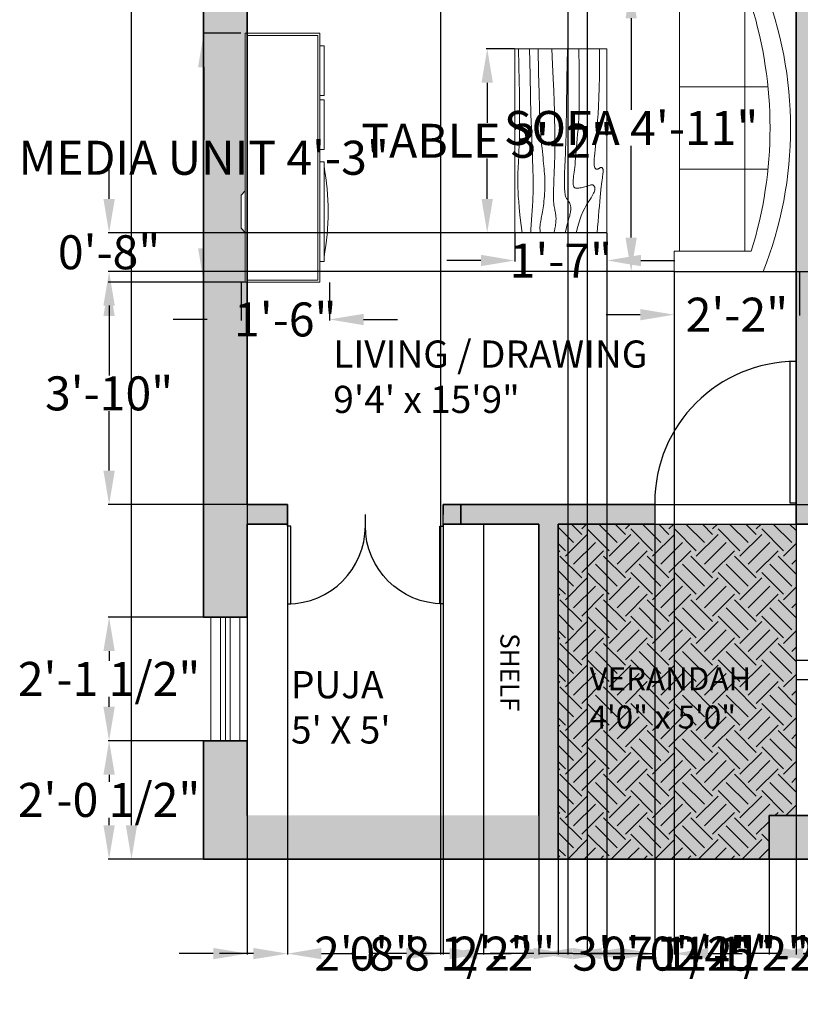
# Model space of a CAD drawing. Units: inches. Extents: x -8 to 329, y 10 to 430.
# Tile 1 of 4: x -8 to 153, y 10 to 213. Entities that reach past the tile are written whole.
import ezdxf

# ---------------------------------------------------------------- set-up
doc = ezdxf.new("R2010")
doc.units = ezdxf.units.IN
doc.header["$MEASUREMENT"] = 0
for name, color, linetype, lineweight in [('A-ANNO-DIMS', 2, 'Continuous', 18), ('A-ANNO-TEXT', 7, 'Continuous', 18), ('A-AREA-IDEN', 7, 'Continuous', 18), ('A-DOOR', 3, 'Continuous', 25), ('A-FLOR-CASE', 9, 'Continuous', 25), ('A-FLOR-STRS', 7, 'Continuous', 25), ('A-FURN', 8, 'Continuous', 18), ('A-GLAZ', 4, 'Continuous', 18), ('A-WALL', 7, 'Continuous', 35), ('A-WALL-PATT', 253, 'Continuous', 13)]:
    doc.layers.add(name, color=color, linetype=linetype, lineweight=lineweight)
doc.layers.add('A-FLOR-BASE-PATT', color=126, linetype='Continuous', lineweight=13, true_color=0x1e6f63)
doc.layers.add('A-FLOR-PATT', color=39, linetype='Continuous', lineweight=13, true_color=0x603913)
doc.styles.get("Standard").update_dxf_attribs({"font": 'arial.ttf'})
doc.dimstyles.get("Standard").update_dxf_attribs({"dimtxt": 7, "dimasz": 7, "dimexe": 0.18, "dimexo": 0.0625, "dimgap": 0.09, "dimtad": 0, "dimtih": 1, "dimtoh": 1, "dimdec": 0, "dimzin": 0, "dimdsep": 46, "dimlunit": 3, "dimtxsty": 'Standard', "dimcen": 0.09, "dimadec": 0, "dimazin": 0, "dimtfac": 1, "dimtdec": 0, "dimtofl": 0, "dimtmove": 0, "dimatfit": 3, "dimfxl": 1, "dimtolj": 1, "dimtzin": 0, "dimarcsym": 0})

# ---------------------------------------------------------------- blocks, each defined once
blk = doc.blocks.new('Sofa - Roundback 7 ft.')
for p, q in [((-12.00002, -32.4421), (-12.00003, -6.5971)), ((11.99997, -32.4421), (11.99998, -6.5971)), ((-36.000027, -34), (-36.000027, -11.4696)), ((35.99998, -34), (35.99998, -11.4696)), ((-35.999844, -13.3819), (35.9998, -13.3819)), ((-36.000027, -32.4421), (35.99998, -32.4421))]:
    blk.add_line(p, q)
for points in [[(-36.000027, -34), (-42.000027, -34), (-42.000027, -8)], [(41.99998, -8), (41.99998, -34), (35.99998, -34)]]:
    blk.add_lwpolyline(points)
for centre, radius, start, end in [((0, -114.25), 114.25, 68.43141, 111.5686), ((-0.00001, -127.1968), 121.1968, 72.72033, 107.2797)]:
    blk.add_arc(centre, radius, start, end)
blk = doc.blocks.new('Entertainment Center')
for p, q in [((-4, 0), (-5, -1)), ((4, 0), (-4, 0)), ((5, -1), (4, 0)), ((-17, -19), (-17, -1)), ((-17, -1), (43, -1)), ((-16.5, -18.5), (-16.5, -1.5)), ((-16.5, -1.5), (42.5, -1.5)), ((42.5, -1.5), (42.5, -18.5)), ((43, -1), (43, -19)), ((42.5, -18.5), (-16.5, -18.5)), ((43, -19), (-17, -19)), ((-12, -20), (-12, -19)), ((12, -20), (-12, -20)), ((12, -19), (12, -20)), ((15, -20), (15, -19)), ((27, -20), (15, -20)), ((27, -19), (27, -20)), ((28, -20), (28, -19)), ((40, -20), (28, -20)), ((40, -19), (40, -20))]:
    blk.add_line(p, q)
blk.add_arc((0, 40), 61, 259.6111, 280.3889)
blk = doc.blocks.new('Table - Rectangular Woodgrain 60 x 30 in.')
for p, q in [((0, 0), (0, -30)), ((60, 0), (0, 0)), ((60, -30), (60, 0)), ((0, -30), (60, -30))]:
    blk.add_line(p, q)
for points in [[(0, -2.4), (4.8155, -2.418), (9.0302, -2.4688), (12.709, -2.5477), (15.9167, -2.65), (18.7181, -2.7711), (21.1781, -2.9063), (23.3616, -3.0508), (25.3333, -3.2), (27.1477, -3.3495), (28.8172, -3.4958), (30.3437, -3.636), (31.7291, -3.7667), (32.9756, -3.8849), (34.0849, -3.9875), (35.059, -4.0714), (35.9, -4.1334), (36.6114, -4.1711), (37.2041, -4.1854), (37.6906, -4.1779), (38.0833, -4.15), (38.3948, -4.1034), (38.6375, -4.0396), (38.8239, -3.9602), (38.9666, -3.8667), (39.0764, -3.7608), (39.1573, -3.6448), (39.2116, -3.521), (39.2416, -3.3917), (39.2498, -3.2593), (39.2385, -3.1261), (39.21, -2.9944), (39.1666, -2.8667), (39.111, -2.7447), (39.0468, -2.6281), (38.978, -2.5163), (38.9083, -2.4083), (38.8418, -2.3035), (38.7823, -2.201), (38.7337, -2.1001), (38.7, -2), (38.6844, -1.9003), (38.6875, -1.8021), (38.7094, -1.707), (38.75, -1.6167), (38.8094, -1.5326), (38.8875, -1.4563), (38.9844, -1.3893), (39.1, -1.3333), (39.2351, -1.2896), (39.3937, -1.2583), (39.5804, -1.2396), (39.8, -1.2333), (40.057, -1.2396), (40.3562, -1.2583), (40.7023, -1.2896), (41.1, -1.3333), (41.5547, -1.3895), (42.0755, -1.4573), (42.6721, -1.5361), (43.3542, -1.625), (44.1316, -1.7233), (45.014, -1.8302), (46.0114, -1.9449), (47.1333, -2.0667), (48.3862, -2.1947), (49.7625, -2.3281), (51.2513, -2.4663), (52.8416, -2.6083), (54.5226, -2.7535), (56.2833, -2.9011), (58.1127, -3.0501), (60, -3.2)], [(0, -9.2), (6.5759, -9.0858), (11.9385, -9.0365), (16.2527, -9.0418), (19.6833, -9.0917), (22.3952, -9.1759), (24.5531, -9.2844), (26.322, -9.4069), (27.8666, -9.5333), (29.3241, -9.6553), (30.7203, -9.7719), (32.0532, -9.8837), (33.3208, -9.9917), (34.5213, -10.0965), (35.6526, -10.199), (36.7128, -10.2999), (37.7, -10.4), (38.6129, -10.4996), (39.4531, -10.5969), (40.223, -10.6895), (40.925, -10.775), (41.5613, -10.8512), (42.1344, -10.9156), (42.6465, -10.966), (43.1, -11), (43.4976, -11.0158), (43.8437, -11.0136), (44.143, -10.9942), (44.4, -10.9583), (44.6195, -10.9069), (44.8062, -10.8406), (44.9648, -10.7603), (45.1, -10.6667), (45.2155, -10.5598), (45.3114, -10.4365), (45.3871, -10.2929), (45.4416, -10.125), (45.4743, -9.929), (45.4844, -9.7011), (45.4709, -9.4371), (45.4333, -9.1333), (45.3716, -8.7883), (45.2896, -8.4104), (45.1919, -8.0107), (45.0833, -7.6), (44.9685, -7.1893), (44.8521, -6.7896), (44.7388, -6.4117), (44.6333, -6.0667), (44.54, -5.7628), (44.4614, -5.4979), (44.4001, -5.2675), (44.3583, -5.0667), (44.3384, -4.8909), (44.3427, -4.7354), (44.3736, -4.5956), (44.4333, -4.4667), (44.5236, -4.3453), (44.6427, -4.2333), (44.7884, -4.1339), (44.9583, -4.05), (45.1501, -3.9849), (45.3614, -3.9417), (45.59, -3.9234), (45.8333, -3.9333), (46.0915, -3.9749), (46.3734, -4.0531), (46.6906, -4.1736), (47.0542, -4.3417), (47.4756, -4.5629), (47.9661, -4.8427), (48.5372, -5.1866), (49.2, -5.6), (49.9676, -6.0844), (50.8594, -6.625), (51.8965, -7.2031), (53.1, -7.8), (54.491, -8.3969), (56.0906, -8.975), (57.9199, -9.5156), (60, -10)], [(0, -12.8), (5.1847, -12.9322), (9.6213, -13.0323), (13.3963, -13.1059), (16.5958, -13.1583), (19.3063, -13.1952), (21.614, -13.2219), (23.6054, -13.2439), (25.3666, -13.2667), (26.9728, -13.2947), (28.4531, -13.3281), (29.8256, -13.3663), (31.1083, -13.4083), (32.3191, -13.4535), (33.476, -13.501), (34.597, -13.5501), (35.7, -13.6), (36.7984, -13.6497), (37.8875, -13.6979), (38.9578, -13.743), (40, -13.7833), (41.0047, -13.8174), (41.9625, -13.8438), (42.864, -13.8607), (43.7, -13.8667), (44.4631, -13.8604), (45.1552, -13.8417), (45.7801, -13.8104), (46.3416, -13.7667), (46.8439, -13.7104), (47.2906, -13.6417), (47.6858, -13.5604), (48.0333, -13.4667), (48.3375, -13.3608), (48.6042, -13.2448), (48.8396, -13.121), (49.05, -12.9917), (49.2417, -12.8593), (49.4208, -12.7261), (49.5937, -12.5944), (49.7667, -12.4667), (49.9452, -12.3451), (50.1323, -12.2313), (50.3303, -12.1268), (50.5416, -12.0333), (50.7686, -11.9524), (51.0135, -11.8854), (51.2788, -11.8341), (51.5666, -11.8), (51.8785, -11.7843), (52.2116, -11.7865), (52.562, -11.8059), (52.926, -11.8417), (53.2998, -11.8931), (53.6795, -11.9594), (54.0614, -12.0397), (54.4416, -12.1333), (54.8223, -12.2401), (55.2293, -12.3625), (55.6942, -12.5037), (56.2489, -12.6667), (56.9251, -12.8547), (57.7545, -13.0708), (58.7689, -13.3182), (60, -13.6)], [(0, -18), (5.124, -17.7273), (9.6609, -17.5057), (13.6705, -17.3303), (17.2125, -17.1958), (20.3467, -17.0973), (23.1328, -17.0297), (25.6307, -16.9878), (27.9, -16.9667), (29.9928, -16.9617), (31.9302, -16.9703), (33.7254, -16.9907), (35.3917, -17.0208), (36.9423, -17.0588), (38.3906, -17.1026), (39.7499, -17.1503), (41.0333, -17.2), (42.2519, -17.2496), (43.4073, -17.2969), (44.4986, -17.3395), (45.525, -17.375), (46.4858, -17.4012), (47.3802, -17.4156), (48.2074, -17.416), (48.9667, -17.4), (49.6583, -17.3662), (50.2872, -17.3167), (50.8595, -17.2547), (51.3812, -17.1833), (51.8584, -17.1057), (52.2971, -17.025), (52.7034, -16.9443), (53.0833, -16.8667), (53.443, -16.7951), (53.789, -16.7313), (54.128, -16.6768), (54.4666, -16.6334), (54.8115, -16.6024), (55.1693, -16.5854), (55.5465, -16.5841), (55.95, -16.6), (56.3828, -16.6337), (56.8346, -16.6823), (57.2915, -16.7418), (57.7396, -16.8084), (58.165, -16.878), (58.5539, -16.9469), (58.8924, -17.0111), (59.1666, -17.0667), (59.3679, -17.1107), (59.5078, -17.1438), (59.6032, -17.1675), (59.6708, -17.1833), (59.7275, -17.193), (59.7901, -17.1979), (59.8753, -17.1998), (60, -17.2)], [(0, -22.4), (8.0098, -22.2501), (14.4094, -22.1011), (19.4168, -21.9535), (23.25, -21.8083), (26.1269, -21.6663), (28.2656, -21.5281), (29.884, -21.3947), (31.2, -21.2667), (32.3967, -21.1448), (33.5172, -21.0292), (34.5697, -20.9198), (35.5625, -20.8167), (36.5037, -20.7198), (37.4015, -20.6292), (38.2642, -20.5448), (39.1, -20.4667), (39.9164, -20.3951), (40.7187, -20.3313), (41.5117, -20.2768), (42.3, -20.2333), (43.0883, -20.2024), (43.8812, -20.1854), (44.6836, -20.1841), (45.5, -20.2), (46.3328, -20.234), (47.1747, -20.2844), (48.0163, -20.3488), (48.8479, -20.425), (49.66, -20.5106), (50.4429, -20.6031), (51.1872, -20.7004), (51.8833, -20.8), (52.5246, -20.8999), (53.1166, -20.9995), (53.6681, -21.0983), (54.1875, -21.1958), (54.6834, -21.2919), (55.1646, -21.3859), (55.6394, -21.4777), (56.1167, -21.5667), (56.6028, -21.6515), (57.0961, -21.7266), (57.5929, -21.7852), (58.0896, -21.8208), (58.5823, -21.8268), (59.0674, -21.7964), (59.5412, -21.723), (60, -21.6)], [(0, -25.2), (8.6355, -25.0504), (15.7026, -24.9031), (21.4049, -24.7606), (25.9458, -24.625), (29.529, -24.4988), (32.3578, -24.3844), (34.6359, -24.284), (36.5667, -24.2), (38.3213, -24.1341), (39.9417, -24.0854), (41.437, -24.0523), (42.8167, -24.0333), (44.0901, -24.0268), (45.2667, -24.0313), (46.3557, -24.0451), (47.3667, -24.0667), (48.309, -24.0947), (49.1928, -24.1287), (50.0284, -24.168), (50.826, -24.2125), (51.5959, -24.2617), (52.3483, -24.3151), (53.0935, -24.3725), (53.8417, -24.4334), (54.6009, -24.497), (55.3699, -24.561), (56.1454, -24.6226), (56.9239, -24.6792), (57.7021, -24.7279), (58.4764, -24.7662), (59.2435, -24.7911), (60, -24.8)], [(0, -28.8), (5.6867, -28.6681), (10.45, -28.5698), (14.407, -28.5012), (17.675, -28.4584), (20.3711, -28.4374), (22.6125, -28.4344), (24.5164, -28.4455), (26.2, -28.4667), (27.762, -28.4947), (29.2276, -28.5281), (30.6033, -28.5663), (31.8958, -28.6084), (33.1118, -28.6535), (34.2578, -28.7011), (35.3405, -28.7501), (36.3666, -28.8), (37.3443, -28.8497), (38.288, -28.8974), (39.2137, -28.9412), (40.1375, -28.9792), (41.0753, -29.0093), (42.0432, -29.0297), (43.0572, -29.0384), (44.1333, -29.0333), (45.2936, -29.0114), (46.5843, -28.9641), (48.0579, -28.8816), (49.7666, -28.7542), (51.7629, -28.5721), (54.0989, -28.3255), (56.8272, -28.0048), (60, -27.6)]]:
    blk.add_lwpolyline(points)
blk = doc.blocks.new('*U11')
for p, q in [((0, 0), (0, 6)), ((40, 0), (40, 6))]:
    blk.add_line(p, q)
blk.add_lwpolyline([(0, 0), (0, -40), (1.75, -40), (1.75, 0)], close=True)
blk.add_arc((0, 0), 40, 270, 0)
blk = doc.blocks.new('*U12')
for p, q in [((0, 0), (0, -6)), ((-40, 0), (-40, -6))]:
    blk.add_line(p, q)
blk.add_lwpolyline([(0, 0), (0, 40), (-1.75, 40), (-1.75, 0)], close=True)
blk.add_arc((0, 0), 40, 90, 180)
blk = doc.blocks.new('*D15')
at = {"layer": 'A-ANNO-DIMS', "color": 0, "lineweight": -2, "transparency": 16777216}
for p, q in [((29.84, 399.76), (14.88, 399.76)), ((15.06, 392.76), (15.06, 223.43)), ((15.06, 46.76), (15.06, 216.1)), ((29.84, 39.76), (14.88, 39.76))]:
    blk.add_line(p, q, dxfattribs=at)
at = {"layer": 'A-ANNO-DIMS', "color": 0, "transparency": 16777216}
for points in [[(13.89, 392.76), (16.23, 392.76), (15.06, 399.76)], [(13.89, 46.76), (16.23, 46.76), (15.06, 39.76)]]:
    blk.add_solid(points, dxfattribs=at)
at = {"layer": 'Defpoints', "color": 0, "transparency": 16777216}
for p in [(29.9, 399.76), (15.06, 39.76), (29.9, 39.76)]:
    blk.add_point(p, dxfattribs=at)
at = {"layer": 'A-ANNO-DIMS', "color": 0, "transparency": 16777216, "insert": (15.06, 219.76), "char_height": 7, "attachment_point": 5}
blk.add_mtext('\\A1;30\'0"', dxfattribs=at)
blk = doc.blocks.new('*D32')
at = {"layer": 'A-ANNO-DIMS', "color": 0, "lineweight": -2, "transparency": 16777216}
for p, q in [((126.75, 219.9), (117.76, 219.9)), ((117.94, 212.9), (117.94, 194.03)), ((117.94, 167.75), (117.94, 186.61)), ((126.75, 160.75), (117.76, 160.75))]:
    blk.add_line(p, q, dxfattribs=at)
at = {"layer": 'A-ANNO-DIMS', "color": 0, "transparency": 16777216}
for points in [[(116.77, 212.9), (119.1, 212.9), (117.94, 219.9)], [(116.77, 167.75), (119.1, 167.75), (117.94, 160.75)]]:
    blk.add_solid(points, dxfattribs=at)
at = {"layer": 'Defpoints', "color": 0, "transparency": 16777216}
for p in [(126.81, 219.9), (117.94, 160.75), (126.81, 160.75)]:
    blk.add_point(p, dxfattribs=at)
at = {"layer": 'A-ANNO-DIMS', "color": 0, "transparency": 16777216, "insert": (117.94, 190.32), "char_height": 7, "attachment_point": 5}
blk.add_mtext('\\A1;SOFA 4\'-11"', dxfattribs=at)
blk = doc.blocks.new('*D33')
at = {"layer": 'A-ANNO-DIMS', "color": 0, "lineweight": -2, "transparency": 16777216}
for p, q in [((126.81, 160.68), (126.81, 151.69)), ((152.63, 160.68), (152.63, 151.69)), ((119.81, 151.87), (112.81, 151.87)), ((159.63, 151.87), (166.63, 151.87))]:
    blk.add_line(p, q, dxfattribs=at)
at = {"layer": 'A-ANNO-DIMS', "color": 0, "transparency": 16777216}
for points in [[(119.81, 153.04), (119.81, 150.71), (126.81, 151.87)], [(159.63, 153.04), (159.63, 150.71), (152.63, 151.87)]]:
    blk.add_solid(points, dxfattribs=at)
at = {"layer": 'Defpoints', "color": 0, "transparency": 16777216}
for p in [(126.81, 160.75), (152.63, 160.75), (152.63, 151.87)]:
    blk.add_point(p, dxfattribs=at)
at = {"layer": 'A-ANNO-DIMS', "color": 0, "transparency": 16777216, "insert": (139.72, 151.87), "char_height": 7, "attachment_point": 5}
blk.add_mtext('\\A1;2\'-2"', dxfattribs=at)
blk = doc.blocks.new('*D34')
at = {"layer": 'A-ANNO-DIMS', "color": 0, "lineweight": -2, "transparency": 16777216}
for p, q in [((37.56, 209.81), (29.75, 209.81)), ((29.93, 202.81), (29.93, 187.86)), ((29.93, 165.57), (29.93, 180.52)), ((37.56, 158.57), (29.75, 158.57))]:
    blk.add_line(p, q, dxfattribs=at)
at = {"layer": 'A-ANNO-DIMS', "color": 0, "transparency": 16777216}
for points in [[(28.77, 202.81), (31.1, 202.81), (29.93, 209.81)], [(28.77, 165.57), (31.1, 165.57), (29.93, 158.57)]]:
    blk.add_solid(points, dxfattribs=at)
at = {"layer": 'Defpoints', "color": 0, "transparency": 16777216}
for p in [(29.93, 209.81), (37.62, 209.81), (37.62, 158.57)]:
    blk.add_point(p, dxfattribs=at)
at = {"layer": 'A-ANNO-DIMS', "color": 0, "transparency": 16777216, "insert": (29.93, 184.19), "char_height": 7, "attachment_point": 5}
blk.add_mtext('\\A1;MEDIA UNIT 4\'-3"', dxfattribs=at)
blk = doc.blocks.new('*D35')
at = {"layer": 'A-ANNO-DIMS', "color": 0, "lineweight": -2, "transparency": 16777216}
for p, q in [((37.62, 158.51), (37.62, 150.71)), ((55.84, 158.51), (55.84, 150.71)), ((30.62, 150.89), (23.62, 150.89)), ((62.84, 150.89), (69.84, 150.89))]:
    blk.add_line(p, q, dxfattribs=at)
at = {"layer": 'A-ANNO-DIMS', "color": 0, "transparency": 16777216}
for points in [[(30.62, 152.05), (30.62, 149.72), (37.62, 150.89)], [(62.84, 152.05), (62.84, 149.72), (55.84, 150.89)]]:
    blk.add_solid(points, dxfattribs=at)
at = {"layer": 'Defpoints', "color": 0, "transparency": 16777216}
for p in [(37.62, 158.57), (55.84, 158.57), (37.62, 150.89)]:
    blk.add_point(p, dxfattribs=at)
at = {"layer": 'A-ANNO-DIMS', "color": 0, "transparency": 16777216, "insert": (46.73, 150.89), "char_height": 7, "attachment_point": 5}
blk.add_mtext('\\A1;1\'-6"', dxfattribs=at)
blk = doc.blocks.new('*D36')
at = {"layer": 'A-ANNO-DIMS', "color": 0, "lineweight": -2, "transparency": 16777216}
for p, q in [((93.93, 206.64), (88.12, 206.64)), ((88.3, 199.64), (88.3, 191.35)), ((88.3, 175.72), (88.3, 184.01)), ((93.93, 168.72), (88.12, 168.72))]:
    blk.add_line(p, q, dxfattribs=at)
at = {"layer": 'A-ANNO-DIMS', "color": 0, "transparency": 16777216}
for points in [[(87.13, 199.64), (89.47, 199.64), (88.3, 206.64)], [(87.13, 175.72), (89.47, 175.72), (88.3, 168.72)]]:
    blk.add_solid(points, dxfattribs=at)
at = {"layer": 'Defpoints', "color": 0, "transparency": 16777216}
for p in [(93.99, 206.64), (88.3, 168.72), (93.99, 168.72)]:
    blk.add_point(p, dxfattribs=at)
at = {"layer": 'A-ANNO-DIMS', "color": 0, "transparency": 16777216, "insert": (88.3, 187.68), "char_height": 7, "attachment_point": 5}
blk.add_mtext('\\A1;TABLE 3\'-2"', dxfattribs=at)
blk = doc.blocks.new('*D37')
at = {"layer": 'A-ANNO-DIMS', "color": 0, "lineweight": -2, "transparency": 16777216}
for p, q in [((93.99, 168.66), (93.99, 162.85)), ((112.95, 168.66), (112.95, 162.85)), ((86.99, 163.03), (79.99, 163.03)), ((119.95, 163.03), (126.95, 163.03))]:
    blk.add_line(p, q, dxfattribs=at)
at = {"layer": 'A-ANNO-DIMS', "color": 0, "transparency": 16777216}
for points in [[(86.99, 164.2), (86.99, 161.86), (93.99, 163.03)], [(119.95, 164.2), (119.95, 161.86), (112.95, 163.03)]]:
    blk.add_solid(points, dxfattribs=at)
at = {"layer": 'Defpoints', "color": 0, "transparency": 16777216}
for p in [(93.99, 168.72), (112.95, 168.72), (112.95, 163.03)]:
    blk.add_point(p, dxfattribs=at)
at = {"layer": 'A-ANNO-DIMS', "color": 0, "transparency": 16777216, "insert": (103.47, 163.03), "char_height": 7, "attachment_point": 5}
blk.add_mtext('\\A1;1\'-7"', dxfattribs=at)
blk = doc.blocks.new('*D44')
at = {"layer": 'A-ANNO-DIMS', "color": 0, "lineweight": -2, "transparency": 16777216}
for p, q in [((122.79, 108.7), (122.79, 20.13)), ((151.9, 108.7), (151.9, 20.13)), ((115.79, 20.31), (108.79, 20.31)), ((158.9, 20.31), (165.9, 20.31))]:
    blk.add_line(p, q, dxfattribs=at)
at = {"layer": 'A-ANNO-DIMS', "color": 0, "transparency": 16777216}
for points in [[(115.79, 21.48), (115.79, 19.15), (122.79, 20.31)], [(158.9, 21.48), (158.9, 19.15), (151.9, 20.31)]]:
    blk.add_solid(points, dxfattribs=at)
at = {"layer": 'Defpoints', "color": 0, "transparency": 16777216}
for p in [(122.79, 108.76), (151.9, 108.76), (151.9, 20.31)]:
    blk.add_point(p, dxfattribs=at)
at = {"layer": 'A-ANNO-DIMS', "color": 0, "transparency": 16777216, "insert": (137.34, 20.31), "char_height": 7, "attachment_point": 5}
blk.add_mtext('\\A1;2\'-5"', dxfattribs=at)
blk = doc.blocks.new('*D45')
at = {"layer": 'A-ANNO-DIMS', "color": 0, "lineweight": -2, "transparency": 16777216}
for p, q in [((47.18, 108.7), (47.18, 20.13)), ((79.25, 108.7), (79.25, 20.13)), ((40.18, 20.31), (33.18, 20.31)), ((86.25, 20.31), (93.25, 20.31))]:
    blk.add_line(p, q, dxfattribs=at)
at = {"layer": 'A-ANNO-DIMS', "color": 0, "transparency": 16777216}
for points in [[(40.18, 21.48), (40.18, 19.15), (47.18, 20.31)], [(86.25, 21.48), (86.25, 19.15), (79.25, 20.31)]]:
    blk.add_solid(points, dxfattribs=at)
at = {"layer": 'Defpoints', "color": 0, "transparency": 16777216}
for p in [(47.18, 108.76), (79.25, 108.76), (79.25, 20.31)]:
    blk.add_point(p, dxfattribs=at)
at = {"layer": 'A-ANNO-DIMS', "color": 0, "transparency": 16777216, "insert": (63.22, 20.31), "char_height": 7, "attachment_point": 5}
blk.add_mtext('\\A1;2\'-8"', dxfattribs=at)
blk = doc.blocks.new('*D46')
at = {"layer": 'A-ANNO-DIMS', "color": 0, "lineweight": -2, "transparency": 16777216}
for p, q in [((38.9, 112.7), (38.9, 20.13)), ((47.18, 112.7), (47.18, 20.13)), ((31.9, 20.31), (24.9, 20.31)), ((54.18, 20.31), (61.18, 20.31))]:
    blk.add_line(p, q, dxfattribs=at)
at = {"layer": 'A-ANNO-DIMS', "color": 0, "transparency": 16777216}
for points in [[(31.9, 21.48), (31.9, 19.15), (38.9, 20.31)], [(54.18, 21.48), (54.18, 19.15), (47.18, 20.31)]]:
    blk.add_solid(points, dxfattribs=at)
at = {"layer": 'Defpoints', "color": 0, "transparency": 16777216}
for p in [(38.9, 112.76), (47.18, 112.76), (47.18, 20.31)]:
    blk.add_point(p, dxfattribs=at)
at = {"layer": 'A-ANNO-DIMS', "color": 0, "transparency": 16777216, "insert": (78.73, 20.31), "char_height": 7, "attachment_point": 5}
blk.add_mtext('\\A1;0\'-8 1/2"', dxfattribs=at)
blk = doc.blocks.new('*D50')
at = {"layer": 'A-ANNO-DIMS', "color": 0, "lineweight": -2, "transparency": 16777216}
for p, q in [((78.68, 302.7), (78.68, 20.13)), ((104.9, 302.7), (104.9, 20.13)), ((71.68, 20.31), (64.68, 20.31)), ((111.9, 20.31), (118.9, 20.31))]:
    blk.add_line(p, q, dxfattribs=at)
at = {"layer": 'A-ANNO-DIMS', "color": 0, "transparency": 16777216}
for points in [[(71.68, 21.48), (71.68, 19.15), (78.68, 20.31)], [(111.9, 21.48), (111.9, 19.15), (104.9, 20.31)]]:
    blk.add_solid(points, dxfattribs=at)
at = {"layer": 'Defpoints', "color": 0, "transparency": 16777216}
for p in [(78.68, 302.76), (104.9, 302.76), (104.9, 20.31)]:
    blk.add_point(p, dxfattribs=at)
at = {"layer": 'A-ANNO-DIMS', "color": 0, "transparency": 16777216, "insert": (91.79, 20.31), "char_height": 7, "attachment_point": 5}
blk.add_mtext('\\A1;2\'-2"', dxfattribs=at)
blk = doc.blocks.new('*D51')
at = {"layer": 'A-ANNO-DIMS', "color": 0, "lineweight": -2, "transparency": 16777216}
for p, q in [((98.9, 48.7), (98.9, 20.13)), ((87.54, 39.7), (87.54, 20.13)), ((80.54, 20.31), (73.54, 20.31)), ((105.9, 20.31), (112.9, 20.31))]:
    blk.add_line(p, q, dxfattribs=at)
at = {"layer": 'A-ANNO-DIMS', "color": 0, "transparency": 16777216}
for points in [[(80.54, 21.48), (80.54, 19.15), (87.54, 20.31)], [(105.9, 21.48), (105.9, 19.15), (98.9, 20.31)]]:
    blk.add_solid(points, dxfattribs=at)
at = {"layer": 'Defpoints', "color": 0, "transparency": 16777216}
for p in [(98.9, 48.76), (87.54, 39.76), (98.9, 20.31)]:
    blk.add_point(p, dxfattribs=at)
at = {"layer": 'A-ANNO-DIMS', "color": 0, "transparency": 16777216, "insert": (133.17, 20.31), "char_height": 7, "attachment_point": 5}
blk.add_mtext('\\A1;0\'-11 1/2"', dxfattribs=at)
blk = doc.blocks.new('*D54')
at = {"layer": 'A-ANNO-DIMS', "color": 0, "lineweight": -2, "transparency": 16777216}
for p, q in [((29.84, 89.59), (10.27, 89.59)), ((10.45, 82.59), (10.45, 80.58)), ((10.45, 71.15), (10.45, 73.16)), ((29.84, 64.15), (10.27, 64.15))]:
    blk.add_line(p, q, dxfattribs=at)
at = {"layer": 'A-ANNO-DIMS', "color": 0, "transparency": 16777216}
for points in [[(9.28, 82.59), (11.62, 82.59), (10.45, 89.59)], [(9.28, 71.15), (11.62, 71.15), (10.45, 64.15)]]:
    blk.add_solid(points, dxfattribs=at)
at = {"layer": 'Defpoints', "color": 0, "transparency": 16777216}
for p in [(29.9, 89.59), (10.45, 64.15), (29.9, 64.15)]:
    blk.add_point(p, dxfattribs=at)
at = {"layer": 'A-ANNO-DIMS', "color": 0, "transparency": 16777216, "insert": (10.45, 76.87), "char_height": 7, "attachment_point": 5}
blk.add_mtext('\\A1;2\'-1 1/2"', dxfattribs=at)
blk = doc.blocks.new('*D61')
at = {"layer": 'A-ANNO-DIMS', "color": 0, "lineweight": -2, "transparency": 16777216}
for p, q in [((29.84, 64.15), (10.27, 64.15)), ((10.45, 57.15), (10.45, 55.66)), ((10.45, 46.76), (10.45, 48.25)), ((29.84, 39.76), (10.27, 39.76))]:
    blk.add_line(p, q, dxfattribs=at)
at = {"layer": 'A-ANNO-DIMS', "color": 0, "transparency": 16777216}
for points in [[(9.28, 57.15), (11.62, 57.15), (10.45, 64.15)], [(9.28, 46.76), (11.62, 46.76), (10.45, 39.76)]]:
    blk.add_solid(points, dxfattribs=at)
at = {"layer": 'Defpoints', "color": 0, "transparency": 16777216}
for p in [(10.45, 64.15), (29.9, 64.15), (29.9, 39.76)]:
    blk.add_point(p, dxfattribs=at)
at = {"layer": 'A-ANNO-DIMS', "color": 0, "transparency": 16777216, "insert": (10.45, 51.96), "char_height": 7, "attachment_point": 5}
blk.add_mtext('\\A1;2\'-0 1/2"', dxfattribs=at)
blk = doc.blocks.new('*D66')
at = {"layer": 'A-ANNO-DIMS', "color": 0, "lineweight": -2, "transparency": 16777216}
for p, q in [((155.9, 48.7), (155.9, 20.13)), ((164.9, 48.7), (164.9, 20.13)), ((148.9, 20.31), (141.9, 20.31)), ((171.9, 20.31), (178.9, 20.31))]:
    blk.add_line(p, q, dxfattribs=at)
at = {"layer": 'A-ANNO-DIMS', "color": 0, "transparency": 16777216}
for points in [[(148.9, 21.48), (148.9, 19.15), (155.9, 20.31)], [(171.9, 21.48), (171.9, 19.15), (164.9, 20.31)]]:
    blk.add_solid(points, dxfattribs=at)
at = {"layer": 'Defpoints', "color": 0, "transparency": 16777216}
for p in [(155.9, 48.76), (164.9, 48.76), (164.9, 20.31)]:
    blk.add_point(p, dxfattribs=at)
at = {"layer": 'A-ANNO-DIMS', "color": 0, "transparency": 16777216, "insert": (188.29, 20.31), "char_height": 7, "attachment_point": 5}
blk.add_mtext('\\A1;0\'-9"', dxfattribs=at)
blk = doc.blocks.new('*D70')
at = {"layer": 'A-ANNO-DIMS', "color": 0, "lineweight": -2, "transparency": 16777216}
for p, q in [((104.9, 306.7), (104.9, 20.13)), ((108.9, 306.7), (108.9, 20.13)), ((97.9, 20.31), (90.9, 20.31)), ((115.9, 20.31), (122.9, 20.31))]:
    blk.add_line(p, q, dxfattribs=at)
at = {"layer": 'A-ANNO-DIMS', "color": 0, "transparency": 16777216}
for points in [[(97.9, 21.48), (97.9, 19.15), (104.9, 20.31)], [(115.9, 21.48), (115.9, 19.15), (108.9, 20.31)]]:
    blk.add_solid(points, dxfattribs=at)
at = {"layer": 'Defpoints', "color": 0, "transparency": 16777216}
for p in [(104.9, 306.76), (108.9, 306.76), (108.9, 20.31)]:
    blk.add_point(p, dxfattribs=at)
at = {"layer": 'A-ANNO-DIMS', "color": 0, "transparency": 16777216, "insert": (132.29, 20.31), "char_height": 7, "attachment_point": 5}
blk.add_mtext('\\A1;0\'-4"', dxfattribs=at)
blk = doc.blocks.new('*D71')
at = {"layer": 'A-ANNO-DIMS', "color": 0, "lineweight": -2, "transparency": 16777216}
for p, q in [((102.9, 39.7), (102.9, 20.13)), ((146.32, 39.7), (146.32, 20.13)), ((95.9, 20.31), (88.9, 20.31)), ((153.32, 20.31), (160.32, 20.31))]:
    blk.add_line(p, q, dxfattribs=at)
at = {"layer": 'A-ANNO-DIMS', "color": 0, "transparency": 16777216}
for points in [[(95.9, 21.48), (95.9, 19.15), (102.9, 20.31)], [(153.32, 21.48), (153.32, 19.15), (146.32, 20.31)]]:
    blk.add_solid(points, dxfattribs=at)
at = {"layer": 'Defpoints', "color": 0, "transparency": 16777216}
for p in [(102.9, 39.76), (146.32, 39.76), (146.32, 20.31)]:
    blk.add_point(p, dxfattribs=at)
at = {"layer": 'A-ANNO-DIMS', "color": 0, "transparency": 16777216, "insert": (124.61, 20.31), "char_height": 7, "attachment_point": 5}
blk.add_mtext('\\A1;3\'-7 1/2"', dxfattribs=at)
blk = doc.blocks.new('*D72')
at = {"layer": 'A-ANNO-DIMS', "color": 0, "lineweight": -2, "transparency": 16777216}
for p, q in [((126.87, 160.75), (289.53, 160.75)), ((289.35, 153.75), (289.35, 140.42)), ((289.35, 119.76), (289.35, 133.09)), ((122.85, 112.76), (289.53, 112.76))]:
    blk.add_line(p, q, dxfattribs=at)
at = {"layer": 'A-ANNO-DIMS', "color": 0, "transparency": 16777216}
for points in [[(288.18, 153.75), (290.52, 153.75), (289.35, 160.75)], [(288.18, 119.76), (290.52, 119.76), (289.35, 112.76)]]:
    blk.add_solid(points, dxfattribs=at)
at = {"layer": 'Defpoints', "color": 0, "transparency": 16777216}
for p in [(126.81, 160.75), (122.79, 112.76), (289.35, 112.76)]:
    blk.add_point(p, dxfattribs=at)
at = {"layer": 'A-ANNO-DIMS', "color": 0, "transparency": 16777216, "insert": (289.35, 136.76), "char_height": 7, "attachment_point": 5}
blk.add_mtext('\\A1;4\'-0"', dxfattribs=at)
blk = doc.blocks.new('*D73')
at = {"layer": 'A-ANNO-DIMS', "color": 0, "lineweight": -2, "transparency": 16777216}
for p, q in [((38.41, 158.57), (10.27, 158.57)), ((10.45, 151.57), (10.45, 139.33)), ((10.45, 119.76), (10.45, 132)), ((38.84, 112.76), (10.27, 112.76))]:
    blk.add_line(p, q, dxfattribs=at)
at = {"layer": 'A-ANNO-DIMS', "color": 0, "transparency": 16777216}
for points in [[(9.28, 151.57), (11.62, 151.57), (10.45, 158.57)], [(9.28, 119.76), (11.62, 119.76), (10.45, 112.76)]]:
    blk.add_solid(points, dxfattribs=at)
at = {"layer": 'Defpoints', "color": 0, "transparency": 16777216}
for p in [(38.47, 158.57), (10.45, 112.76), (38.9, 112.76)]:
    blk.add_point(p, dxfattribs=at)
at = {"layer": 'A-ANNO-DIMS', "color": 0, "transparency": 16777216, "insert": (10.45, 135.67), "char_height": 7, "attachment_point": 5}
blk.add_mtext('\\A1;3\'-10"', dxfattribs=at)
blk = doc.blocks.new('*D74')
at = {"layer": 'A-ANNO-DIMS', "color": 0, "lineweight": -2, "transparency": 16777216}
for p, q in [((112.95, 168.66), (112.95, 20.13)), ((126.81, 160.68), (126.81, 20.13)), ((105.95, 20.31), (98.95, 20.31)), ((133.81, 20.31), (140.81, 20.31))]:
    blk.add_line(p, q, dxfattribs=at)
at = {"layer": 'A-ANNO-DIMS', "color": 0, "transparency": 16777216}
for points in [[(105.95, 21.48), (105.95, 19.15), (112.95, 20.31)], [(133.81, 21.48), (133.81, 19.15), (126.81, 20.31)]]:
    blk.add_solid(points, dxfattribs=at)
at = {"layer": 'Defpoints', "color": 0, "transparency": 16777216}
for p in [(112.95, 168.72), (126.81, 160.75), (126.81, 20.31)]:
    blk.add_point(p, dxfattribs=at)
at = {"layer": 'A-ANNO-DIMS', "color": 0, "transparency": 16777216, "insert": (149.87, 20.31), "char_height": 7, "attachment_point": 5}
blk.add_mtext('\\A1;1\'-2"', dxfattribs=at)
blk = doc.blocks.new('*D75')
at = {"layer": 'A-ANNO-DIMS', "color": 0, "lineweight": -2, "transparency": 16777216}
for p, q in [((10.45, 175.72), (10.45, 182.72)), ((112.89, 168.72), (10.27, 168.72)), ((126.75, 160.75), (10.27, 160.75)), ((10.45, 153.75), (10.45, 146.75))]:
    blk.add_line(p, q, dxfattribs=at)
at = {"layer": 'A-ANNO-DIMS', "color": 0, "transparency": 16777216}
for points in [[(9.28, 175.72), (11.62, 175.72), (10.45, 168.72)], [(9.28, 153.75), (11.62, 153.75), (10.45, 160.75)]]:
    blk.add_solid(points, dxfattribs=at)
at = {"layer": 'Defpoints', "color": 0, "transparency": 16777216}
for p in [(112.95, 168.72), (10.45, 160.75), (126.81, 160.75)]:
    blk.add_point(p, dxfattribs=at)
at = {"layer": 'A-ANNO-DIMS', "color": 0, "transparency": 16777216, "insert": (10.45, 164.73), "char_height": 7, "attachment_point": 5}
blk.add_mtext('\\A1;0\'-8"', dxfattribs=at)

msp = doc.modelspace()

# ---------------------------------------------------------------- hatches: boundary and pattern name
at = {"layer": 'A-FLOR-BASE-PATT'}
h = msp.add_hatch(color=256, dxfattribs=at)
h.dxf.hatch_style = 1
h.paths.add_polyline_path([(102.9, 48.76), (102.9, 39.76), (146.32, 39.76), (146.32, 48.76), (151.9, 48.76), (151.9, 108.76), (122.79, 108.76), (102.9, 108.76)])
h.paths.add_polyline_path([(108.11, 64.07), (147.28, 64.07), (147.28, 81.73), (108.11, 81.73)], flags=24)
at = {"layer": 'A-FLOR-PATT'}
h = msp.add_hatch(dxfattribs=at)
h.set_pattern_fill('EARTH', color=256, angle=45)
h.set_pattern_definition([(45, (0, 0), (0, 8.98026), [6.35, -6.35]), (45, (-1.684, 1.684), (0, 8.98026), [6.35, -6.35]), (45, (-3.3676, 3.3676), (0, 8.98026), [6.35, -6.35]), (135, (-3.3676, 4.49), (-8.98026, 0), [6.35, -6.35]), (135, (-1.684, 6.174), (-8.98026, 0), [6.35, -6.35]), (135, (0, 7.858), (-8.98026, 0), [6.35, -6.35])])
h.paths.add_polyline_path([(102.9, 48.76), (102.9, 39.76), (146.32, 39.76), (146.32, 48.76), (151.9, 48.76), (151.9, 108.76), (122.79, 108.76), (102.9, 108.76)])
h.paths.add_polyline_path([(108.11, 64.07), (147.28, 64.07), (147.28, 81.73), (108.11, 81.73)], flags=24)
at = {"layer": 'A-WALL-PATT'}
h = msp.add_hatch(color=256, dxfattribs=at)
h.dxf.hatch_style = 1
h.paths.add_polyline_path([(146.32, 48.76), (146.32, 39.76), (269.9, 39.76), (269.9, 145.31), (260.9, 145.31), (260.9, 112.76), (186.22, 112.76), (155.9, 112.76), (155.9, 222.76), (155.9, 239.44), (153.1, 239.44), (151.9, 239.44), (151.9, 222.76), (151.9, 108.76), (260.9, 108.76), (260.9, 48.76)])
h = msp.add_hatch(color=256, dxfattribs=at)
h.dxf.hatch_style = 1
h.paths.add_polyline_path([(38.9, 158.57), (38.47, 158.57), (38.47, 168.82), (37.62, 169.67), (37.62, 176.5), (38.47, 177.36), (38.47, 209.81), (38.9, 209.81), (38.9, 219.28), (29.9, 219.28), (29.9, 89.59), (38.9, 89.59), (38.9, 108.76), (47.18, 108.76), (47.18, 110.76), (47.18, 112.76), (38.9, 112.76)])
h = msp.add_hatch(color=256, dxfattribs=at)
h.dxf.hatch_style = 1
h.paths.add_polyline_path([(38.9, 48.76), (38.9, 64.15), (29.9, 64.15), (29.9, 39.76), (102.9, 39.76), (102.9, 48.76), (102.9, 108.76), (122.79, 108.76), (122.79, 112.76), (102.9, 112.76), (82.84, 112.76), (82.84, 108.76), (98.9, 108.76), (98.9, 48.76)])
h = msp.add_hatch(color=256, dxfattribs=at)
h.dxf.hatch_style = 1
h.paths.add_polyline_path([(79.25, 110.76), (79.25, 108.76), (82.84, 108.76), (82.84, 112.76), (79.25, 112.76)])

# ---------------------------------------------------------------- linework, layer by layer
at = {"layer": 'A-DOOR'}
msp.add_line((122.79, 108.76), (151.9, 108.76), dxfattribs=at)
at = {"layer": 'A-FLOR-CASE'}
msp.add_line((87.54, 108.76), (87.54, 39.76), dxfattribs=at)
at = {"layer": 'A-FLOR-STRS'}
for p, q in [((151.9, 80.76), (151.9, 76.76)), ((151.9, 80.76), (236.56, 80.76)), ((151.9, 76.76), (236.56, 76.76))]:
    msp.add_line(p, q, dxfattribs=at)
at = {"layer": 'A-GLAZ'}
for p, q in [((31.4, 89.59), (31.4, 64.15)), ((33.4, 89.59), (33.4, 64.15)), ((34.4, 89.59), (34.4, 64.15)), ((35.4, 89.59), (35.4, 64.15)), ((37.4, 89.59), (37.4, 64.15))]:
    msp.add_line(p, q, dxfattribs=at)
at = {"layer": 'A-WALL'}
for p, q in [((151.9, 222.76), (151.9, 108.76)), ((29.9, 89.59), (29.9, 219.28)), ((38.9, 112.76), (38.9, 219.28)), ((38.9, 112.76), (47.18, 112.76)), ((47.18, 108.76), (47.18, 112.76)), ((79.25, 112.76), (102.9, 112.76)), ((79.25, 110.76), (79.25, 112.76)), ((82.84, 108.76), (82.84, 112.76)), ((102.9, 112.76), (122.79, 112.76)), ((38.9, 108.76), (47.18, 108.76)), ((38.9, 89.59), (38.9, 108.76)), ((79.25, 108.76), (98.9, 108.76)), ((98.9, 48.76), (98.9, 108.76)), ((102.9, 48.76), (102.9, 108.76)), ((102.9, 108.76), (122.79, 108.76)), ((151.9, 108.76), (260.9, 108.76)), ((38.9, 89.59), (29.9, 89.59)), ((29.9, 39.76), (29.9, 64.15)), ((38.9, 64.15), (29.9, 64.15)), ((38.9, 48.76), (38.9, 64.15)), ((102.9, 48.76), (102.9, 39.76)), ((146.32, 48.76), (260.9, 48.76)), ((146.32, 39.76), (146.32, 48.76)), ((29.9, 39.76), (269.9, 39.76))]:
    msp.add_line(p, q, dxfattribs=at)

# ---------------------------------------------------------------- block references
at = {"layer": 'A-DOOR'}
for name, p, xscale, yscale, zscale in [('*U12', (151.9, 113.13), 0.7278016213330712, 0.7278016213330712, 0.7278016213330712), ('*U11', (47.18, 108.36), 0.4008560385274677, 0.4008560385274677, 0.4008560385274677), ('*U11', (79.25, 108.36), -0.4008560385274677, 0.4008560385274677, 0.4008560385274677)]:
    msp.add_blockref(name, p, dxfattribs=dict(at, xscale=xscale, yscale=yscale, zscale=zscale))
at = {"layer": 'A-FURN'}
for name, p, xscale, yscale, zscale, rotation in [('Sofa - Roundback 7 ft.', (150.75, 190.32), 0.704182813737638, 0.704182813737638, 0.704182813737638, 270), ('Entertainment Center', (37.62, 173.09), 0.8539499527630571, 0.8539499527630571, 0.8539499527630571, 90), ('Table - Rectangular Woodgrain 60 x 30 in.', (112.95, 206.64), 0.6319894406840288, 0.6319894406840288, 0.6319894406840288, 270)]:
    msp.add_blockref(name, p, dxfattribs=dict(at, xscale=xscale, yscale=yscale, zscale=zscale, rotation=rotation))

# ---------------------------------------------------------------- texts
at = {"layer": 'A-ANNO-TEXT', "insert": (94.94, 86.29), "char_height": 3.921, "attachment_point": 1, "rotation": 270}
msp.add_mtext_dynamic_manual_height_columns('SHELF ', width=365.4317, gutter_width=19.61, heights=[5.05], dxfattribs=at)
at = {"layer": 'A-AREA-IDEN', "attachment_point": 1}
for s, width, gutter_width, insert, char_height in [('LIVING / DRAWING\\P9\'4\' x 15\'9"', 164.8422, 27.98, (56.61, 146.56), 5.5954), ('VERANDAH\\P4\'0" x 5\'0"', 139.4594, 23.67, (109.38, 79.29), 4.7338), ("PUJA\\P5' X 5'", 164.8422, 27.98, (47.9, 78.49), 5.595)]:
    msp.add_mtext_dynamic_manual_height_columns(s, width=width, gutter_width=gutter_width, heights=[0], dxfattribs=dict(at, insert=insert, char_height=char_height))

# ---------------------------------------------------------------- dimensions: what is measured, and where the dimension line sits
at = {"layer": 'A-ANNO-DIMS'}
for base, p1, p2, angle, text, override, picture, middle in [((15.06, 39.76), (29.9, 399.76), (29.9, 39.76), 90, '<>0"', {"dimclrd": 0, "dimclre": 0, "dimclrt": 0}, '*D15', (15.06, 219.76)), ((117.9359, 160.747), (126.8086, 219.8983), (126.8086, 160.747), 270, 'SOFA <>', {"dimdec": 1, "dimlfac": 1, "dimrnd": 0, "dimzin": 1, "dimdsep": 46, "dimlunit": 4, "dimfrac": 2}, '*D32', (117.9359, 190.3227)), ((29.93, 209.81), (37.62, 158.57), (37.62, 209.81), 90, 'MEDIA UNIT <>', {"dimdec": 1, "dimlfac": 1, "dimrnd": 0, "dimzin": 1, "dimdsep": 46, "dimlunit": 4, "dimfrac": 2}, '*D34', (29.93, 184.19)), ((88.3, 168.72), (93.99, 206.64), (93.99, 168.72), 270, 'TABLE <>', {"dimdec": 1, "dimlfac": 1, "dimrnd": 0, "dimzin": 1, "dimdsep": 46, "dimlunit": 4, "dimfrac": 2}, '*D36', (88.3, 187.68))]:
    dim = msp.add_linear_dim(base=base, p1=p1, p2=p2, angle=angle, text=text, dimstyle='Standard', override=override, dxfattribs=at)
    dim.commit()
    dim.dimension.update_dxf_attribs({"geometry": picture, "text_midpoint": middle})
for base, p1, p2, picture, middle in [((108.9, 20.31), (104.9, 306.76), (108.9, 306.76), '*D70', (132.29, 20.31)), ((104.9, 20.31), (78.68, 302.76), (104.9, 302.76), '*D50', (91.79, 20.31)), ((112.95, 163.03), (93.99, 168.72), (112.95, 168.72), '*D37', (103.47, 163.03)), ((126.81, 20.31), (112.95, 168.72), (126.81, 160.75), '*D74', (149.87, 20.31)), ((152.63, 151.87), (126.81, 160.75), (152.63, 160.75), '*D33', (139.72, 151.87)), ((47.18, 20.31), (38.9, 112.76), (47.18, 112.76), '*D46', (78.73, 20.31)), ((79.25, 20.31), (47.18, 108.76), (79.25, 108.76), '*D45', (63.22, 20.31)), ((151.9, 20.31), (122.79, 108.76), (151.9, 108.76), '*D44', (137.34, 20.31)), ((98.9, 20.31), (87.54, 39.76), (98.9, 48.76), '*D51', (133.17, 20.31)), ((164.9, 20.31), (155.9, 48.76), (164.9, 48.76), '*D66', (188.29, 20.31)), ((146.32, 20.31), (102.9, 39.76), (146.32, 39.76), '*D71', (124.61, 20.31))]:
    dim = msp.add_linear_dim(base=base, p1=p1, p2=p2, dimstyle='Standard', override={"dimdec": 1, "dimlfac": 1, "dimrnd": 0, "dimzin": 1, "dimdsep": 46, "dimlunit": 4, "dimfrac": 2}, dxfattribs=at)
    dim.commit()
    dim.dimension.update_dxf_attribs({"geometry": picture, "text_midpoint": middle})
for base, p1, p2, angle, picture, middle in [((10.45, 160.75), (112.95, 168.72), (126.81, 160.75), 90, '*D75', (10.45, 164.73)), ((289.35, 112.76), (126.81, 160.75), (122.79, 112.76), 90, '*D72', (289.35, 136.76)), ((10.45, 112.76), (38.47, 158.57), (38.9, 112.76), 90, '*D73', (10.45, 135.67)), ((37.62, 150.89), (55.84, 158.57), (37.62, 158.57), 180, '*D35', (46.73, 150.89)), ((10.45, 64.15), (29.9, 89.59), (29.9, 64.15), 90, '*D54', (10.45, 76.87)), ((10.45, 64.15), (29.9, 39.76), (29.9, 64.15), 90, '*D61', (10.45, 51.96))]:
    dim = msp.add_linear_dim(base=base, p1=p1, p2=p2, angle=angle, dimstyle='Standard', override={"dimdec": 1, "dimlfac": 1, "dimrnd": 0, "dimzin": 1, "dimdsep": 46, "dimlunit": 4, "dimfrac": 2}, dxfattribs=at)
    dim.commit()
    dim.dimension.update_dxf_attribs({"geometry": picture, "text_midpoint": middle})

doc.saveas('drawing.dxf')
